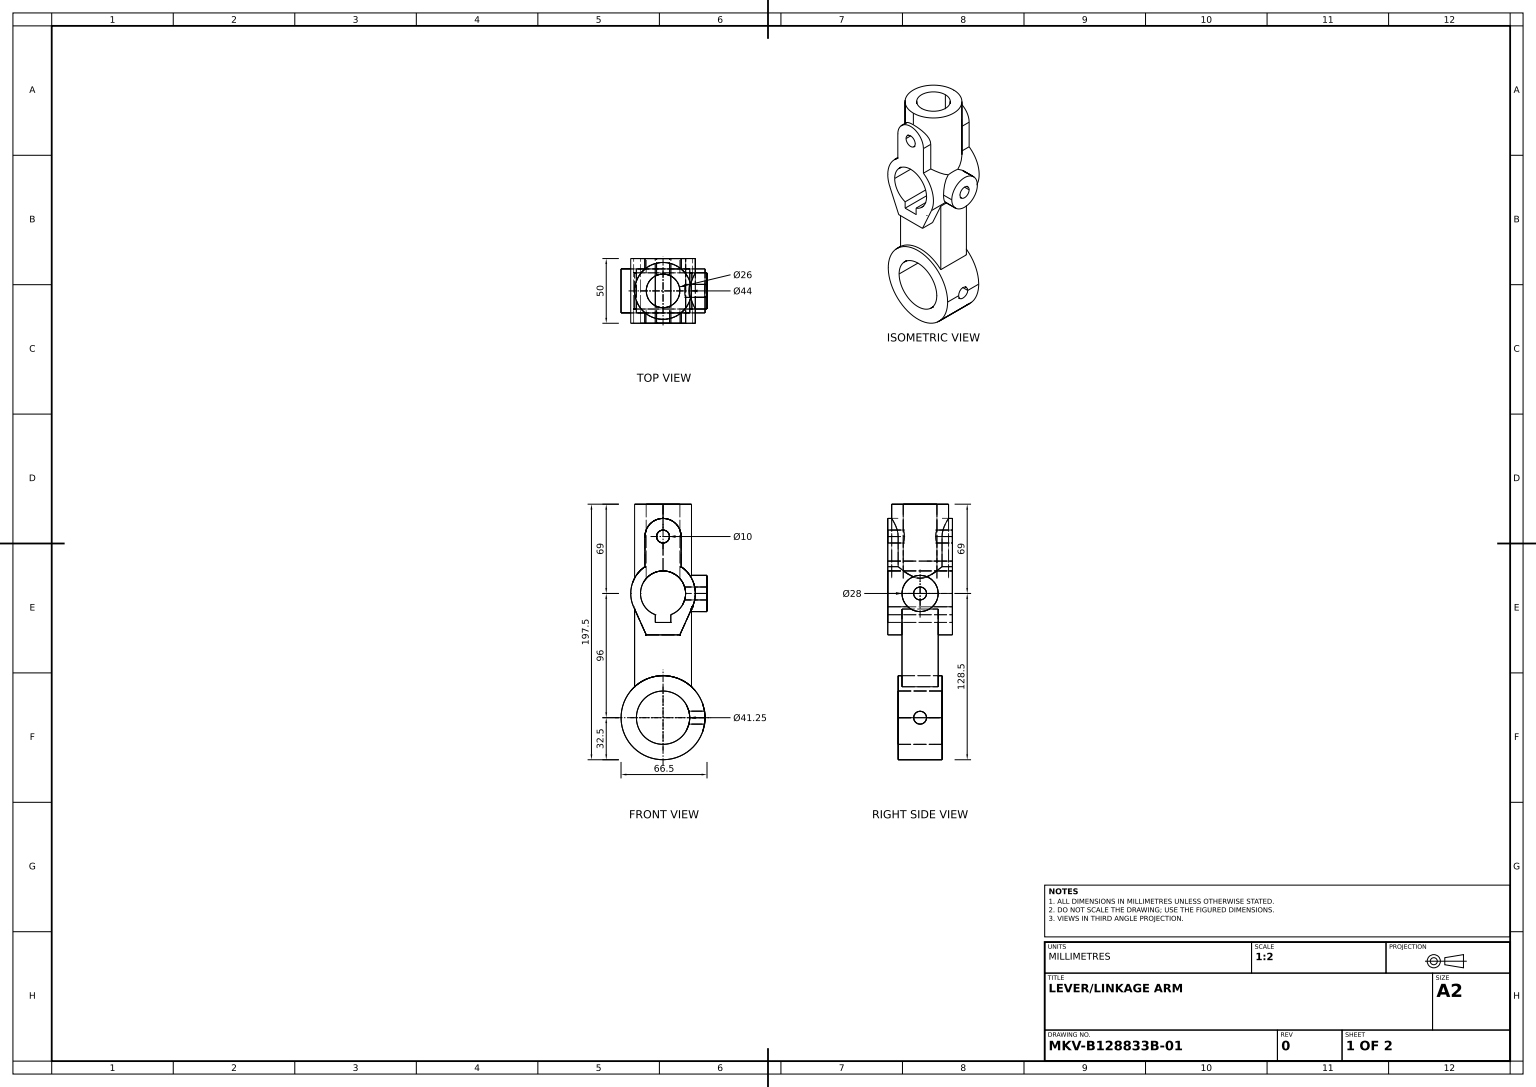
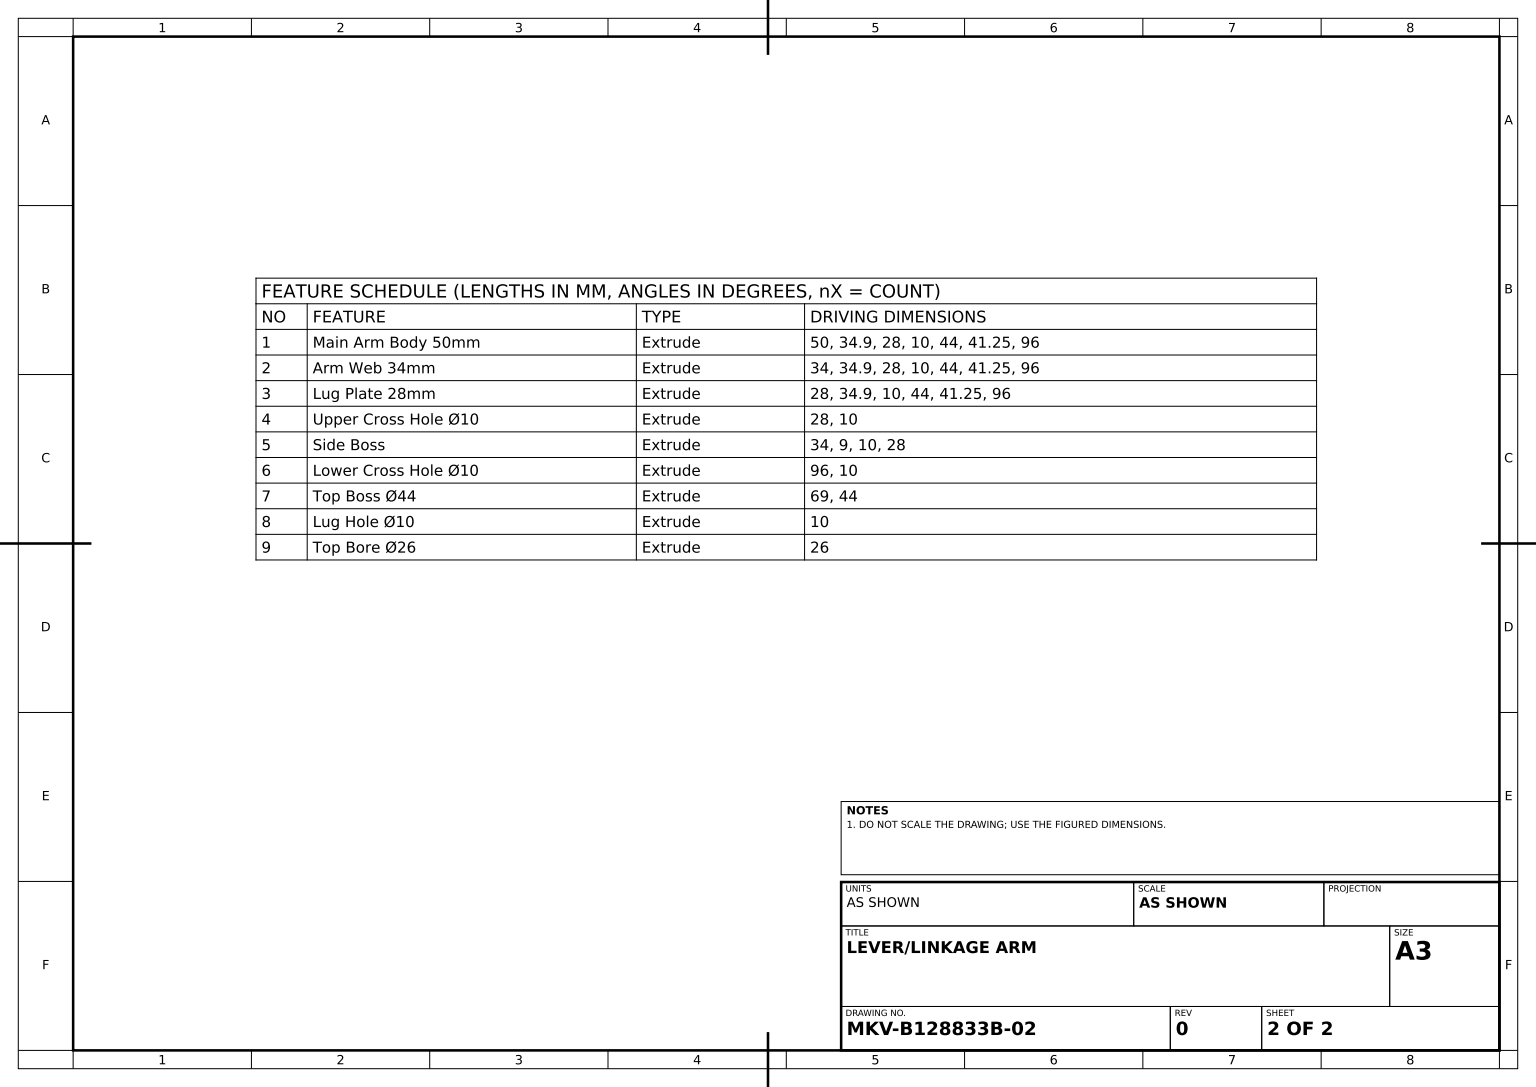
from build123d import *

# Parameters (mm, degrees)
LINK_ARM_PROFILE_SKETCH_R    = 5
MAIN_ARM_BODY_50MM_DEPTH     = 25
SKETCH1_3_R                  = 32.5
SKETCH1_3_R_2                = 20.625
ARM_WEB_34MM_DEPTH           = 17
LUG_PLATE_28MM_DEPTH         = 14
UPPER_CROSS_HOLE_10_SKETCH_R = 5
UPPER_CROSS_HOLE_10_DEPTH    = 28
SIDE_BOSS_REACH              = 148.832
SIDE_BOSS_SKETCH_R           = 14
SIDE_BOSS_SKETCH_R_2         = 5
LOWER_CROSS_HOLE_10_SKETCH_R = 5
LOWER_CROSS_HOLE_10_DEPTH    = 136.252541609
TOP_BOSS_44_REACH            = 203.959
TOP_BOSS_44_END_RADIUS       = 25
TOP_BOSS_44_SKETCH_R         = 22
LUG_HOLE_10_SKETCH_R         = 5
LUG_HOLE_10_DEPTH            = 143.01496415
TOP_BORE_26_REACH            = 203.959
TOP_BORE_26_END_RADIUS       = 17.45
TOP_BORE_26_SKETCH_R         = 13


with BuildPart() as part:
    # Link Arm Profile Sketch → Main Arm Body 50mm (new, symmetric)
    # profile 1 of 2: a face of its own
    with BuildSketch(Plane.XY):
        with BuildLine():
            Line((-14, 44), (-14, 20.712315177))
            ThreePointArc((-14, 20.712315177), (0, 25), (14, 20.712315177))
            Line((14, 20.712315177), (14, 44))
            ThreePointArc((14, 44), (0, 58), (-14, 44))
        make_face()
        with Locations((0, 44)):
            Circle(LINK_ARM_PROFILE_SKETCH_R, mode=Mode.SUBTRACT)
    # profile 2 of 2: a face of its own
    with BuildSketch(Plane.XY):
        with BuildLine():
            ThreePointArc((22.792288735, -10.271882702), (0, 25), (-22.792288735, -10.271882702))
            Line((-22.792288735, -10.271882702), (-13, -32))
            Line((-13, -32), (13, -32))
            Line((13, -32), (22.792288735, -10.271882702))
        make_face()
        with BuildLine():
            ThreePointArc((6, -16.386045893), (0, 17.45), (-6, -16.386045893))
            Line((-6, -16.386045893), (-6, -22.39))
            Line((-6, -22.39), (6, -22.39))
            Line((6, -22.39), (6, -16.386045893))
        make_face(mode=Mode.SUBTRACT)
    extrude(amount=MAIN_ARM_BODY_50MM_DEPTH, both=True)



with BuildPart() as body_2:
    # Sketch1_3 → Arm Web 34mm (new, symmetric)
    with BuildSketch(Plane.XY):
        with Locations((0, -96)):
            Circle(SKETCH1_3_R)
        with Locations((0, -96)):
            Circle(SKETCH1_3_R_2, mode=Mode.SUBTRACT)
    extrude(amount=ARM_WEB_34MM_DEPTH, both=True)


with BuildPart() as part_1:
    add(part.part)

    add(body_2.part)  # Lug Plate 28mm merges body 2
    # Sketch1_5 → Lug Plate 28mm (add, symmetric)
    with BuildSketch(Plane.XY):
        with BuildLine():
            Line((13, -32), (-13, -32))
            Line((-13, -32), (-22, -12.029892808))
            Line((-22, -12.029892808), (-22, -72.078252572))
            ThreePointArc((-22, -72.078252572), (0, -63.5), (22, -72.078252572))
            Line((22, -72.078252572), (22, -12.029892808))
            Line((22, -12.029892808), (13, -32))
        make_face()
    extrude(amount=LUG_PLATE_28MM_DEPTH, both=True)

    # Upper Cross Hole _10 Sketch → Upper Cross Hole _10 (cut)
    with BuildSketch(Plane(origin=(0, 0, 0), x_dir=(0, 0, -1), z_dir=(1, 0, 0))):
        with Locations(Location((0, 0, 0), (0, 0, 180))):
            Circle(UPPER_CROSS_HOLE_10_SKETCH_R)
    extrude(amount=UPPER_CROSS_HOLE_10_DEPTH, mode=Mode.SUBTRACT)

    # Side Boss Sketch → Side Boss (add, up to next)
    with BuildSketch(Plane(origin=(34, 0, 0), x_dir=(0, 0, -1), z_dir=(1, 0, 0)), mode=Mode.PRIVATE) as side_boss_sk1:
        Circle(SIDE_BOSS_SKETCH_R)
        with Locations(Location((0, 0, 0), (0, 0, 180))):
            Circle(SIDE_BOSS_SKETCH_R_2, mode=Mode.SUBTRACT)
    side_boss_tool1 = extrude(side_boss_sk1.sketch, amount=-SIDE_BOSS_REACH, mode=Mode.PRIVATE) - part_1.part
    add(side_boss_tool1.solids().sort_by_distance((34, 0, 13.60402))[0])

    # Lower Cross Hole _10 Sketch → Lower Cross Hole _10 (cut, through all)
    with BuildSketch(Plane(origin=(0, 0, 0), x_dir=(0, 0, -1), z_dir=(1, 0, 0))):
        with Locations(Location((0, -96, 0), (0, 0, 180))):
            Circle(LOWER_CROSS_HOLE_10_SKETCH_R)
    extrude(amount=LOWER_CROSS_HOLE_10_DEPTH, mode=Mode.SUBTRACT)

    # Top Boss _44: up to this cylinder (the profile starts outside it)
    top_boss_44_end = Plane(origin=(0, 0, 0), z_dir=(0, 0, -1)) * Cylinder(TOP_BOSS_44_END_RADIUS, 458.918, mode=Mode.PRIVATE)
    # Top Boss _44 Sketch → Top Boss _44 (add, up to the surface)
    with BuildSketch(Plane(origin=(0, 69, 0), x_dir=(1, 0, 0), z_dir=(0, 1, 0)), mode=Mode.PRIVATE) as top_boss_44_sk1:
        with Locations(Location((0, 0, 0), (0, 0, 270))):
            Circle(TOP_BOSS_44_SKETCH_R)
    top_boss_44_tool1 = extrude(top_boss_44_sk1.sketch, amount=-TOP_BOSS_44_REACH, mode=Mode.PRIVATE) - top_boss_44_end
    add(top_boss_44_tool1.solids().sort_by_distance((0, 69, 0))[0])

    # Lug Hole _10 Sketch → Lug Hole _10 (cut, through all)
    with BuildSketch(Plane.XY.offset(25)):
        with Locations((0, 44)):
            Circle(LUG_HOLE_10_SKETCH_R)
    extrude(amount=-LUG_HOLE_10_DEPTH, mode=Mode.SUBTRACT)

    # Top Bore _26: up to this cylinder (the profile starts outside it)
    top_bore_26_end = Plane(origin=(0, 0, 0), z_dir=(0, 0, -1)) * Cylinder(TOP_BORE_26_END_RADIUS, 443.818, mode=Mode.PRIVATE)
    # Top Bore _26 Sketch → Top Bore _26 (cut, up to the surface)
    with BuildSketch(Plane(origin=(0, 69, 0), x_dir=(1, 0, 0), z_dir=(0, 1, 0)), mode=Mode.PRIVATE) as top_bore_26_sk1:
        with Locations(Location((0, 0, 0), (0, 0, 270))):
            Circle(TOP_BORE_26_SKETCH_R)
    top_bore_26_tool1 = extrude(top_bore_26_sk1.sketch, amount=-TOP_BORE_26_REACH, mode=Mode.PRIVATE) - top_bore_26_end
    add(top_bore_26_tool1.solids().sort_by_distance((0, 69, 0))[0], mode=Mode.SUBTRACT)


solid = part_1.part
